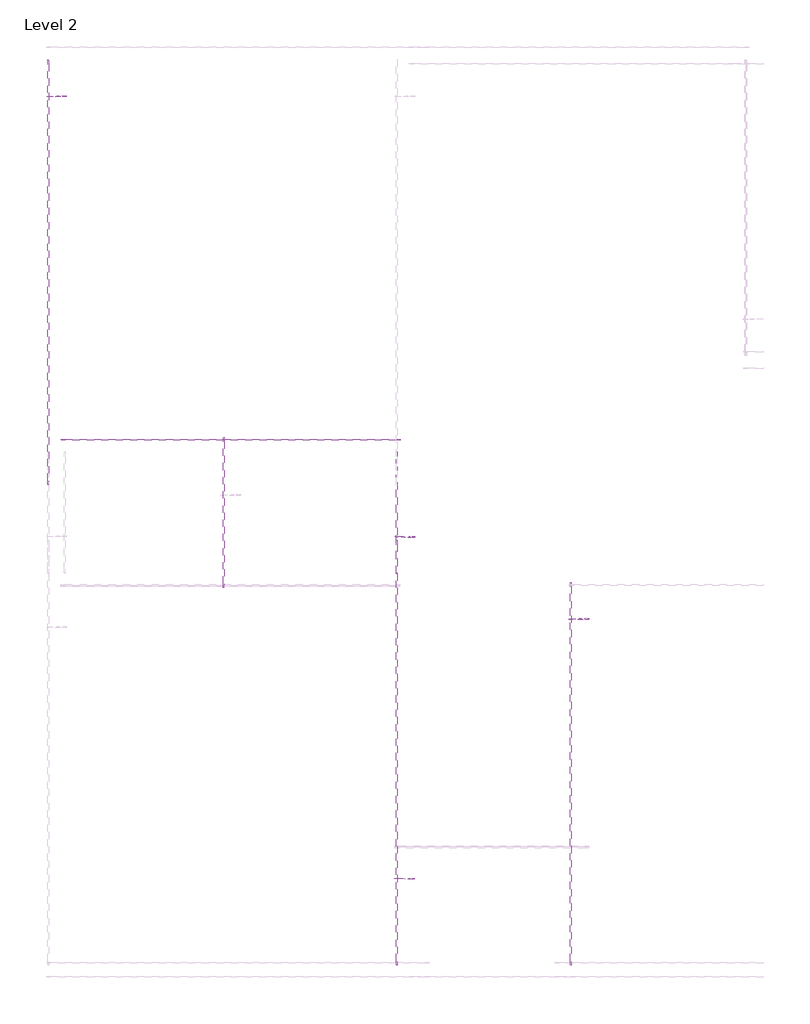
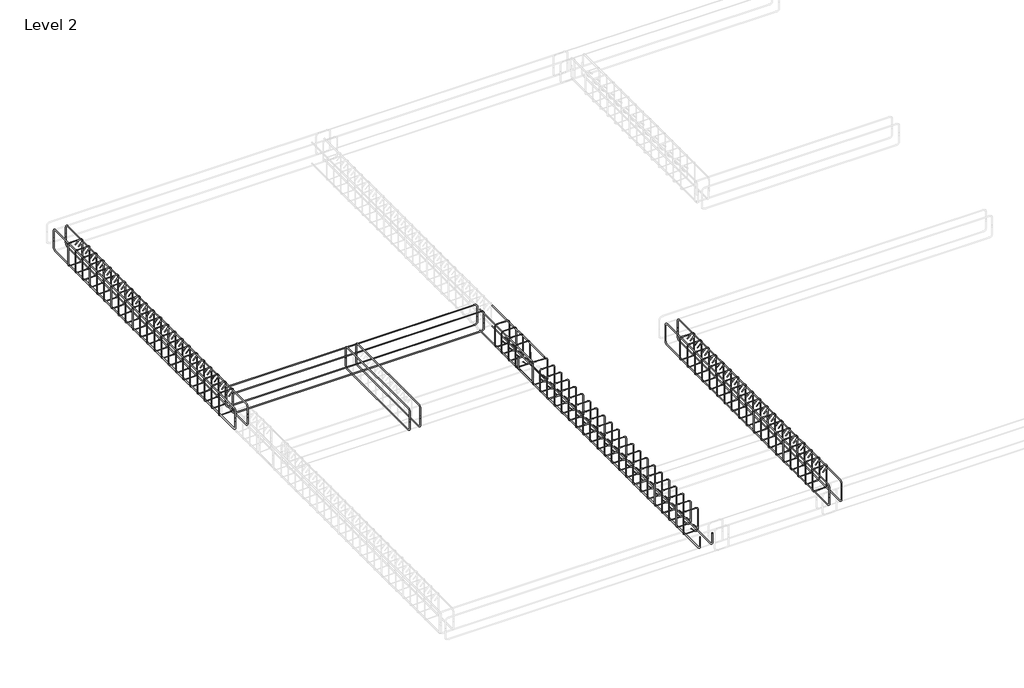
# One storey, part 3 of 5: 15 reinforcing bars.
"""IFC4 building model written with IfcOpenShell, lengths in millimetres."""

from ifc_helpers import new_model, si_unit, point, frame, origin, place, context, project, spatial, polyline, circle_curve, trimmed, segment, composite_curve, source, transform, mapped, element, save
from ifc_brep_helpers import swept_disk

model = new_model("IFC4")

# Units and contexts
model_context = context("Model", 3, world=origin())
ifc_project = project(units=[si_unit("LENGTHUNIT", "METRE", prefix="MILLI")], contexts=[model_context])

# Site, building, storey
site = spatial("IfcSite", under=ifc_project)
building = spatial("IfcBuilding", under=site)
storey = spatial("IfcBuildingStorey", under=building, Name="Level 2", Elevation=3048.0)

# Reinforcing bars
placement = place(None, origin())
reinforcing_bar_shape = source(origin(), model_context, "Body", "SolidModel", [
    swept_disk(composite_curve([segment(polyline([(-15212.455746, 8321.0577522, 5841.8967919), (-15212.455746, 8321.0577522, 5994.2967919)]), True, "CONTINUOUS"), segment(trimmed(circle_curve(frame((-15212.455746, 8276.9887522, 5994.2967919), z_axis=(1.0, 0.0, 0.0), x_axis=(0.0, 44.068999999999505, 0.0)), 44.069), [point((-15212.455746, 8321.0577522, 5994.2967919))], [point((-15212.455746, 8276.9887522, 6038.3657919))], True, "CARTESIAN"), True, "CONTINUOUS"), segment(polyline([(-15212.455746, 8276.9887522, 6038.3657919), (-15212.455746, 3496.0647522, 6038.3657919)]), True, "CONTINUOUS"), segment(trimmed(circle_curve(frame((-15212.455746, 3496.0647522, 5994.2967919), z_axis=(1.0, 0.0, 0.0), x_axis=(0.0, 0.0, 44.068999999999505)), 44.069), [point((-15212.455746, 3496.0647522, 6038.3657919))], [point((-15212.455746, 3451.9957522, 5994.2967919))], True, "CARTESIAN"), True, "CONTINUOUS"), segment(polyline([(-15212.455746, 3451.9957522, 5994.2967919), (-15212.455746, 3451.9957522, 5841.8967919)]), True, "CONTINUOUS")], self_intersect=False), 5.969),
])
element("IfcReinforcingBar", 1, at=placement, inside=storey, context=model_context, shape_type="MappedRepresentation", body=[
    mapped(reinforcing_bar_shape, transform((0.0, 0.0, 0.0), x_axis=(1.0, 0.0, 0.0), y_axis=(0.0, 1.0, 0.0), z_axis=(0.0, 0.0, 1.0))),
    mapped(reinforcing_bar_shape, transform((-189.5315837, 0.0, 0.0), x_axis=(1.0, 0.0, 0.0), y_axis=(0.0, 1.0, 0.0), z_axis=(0.0, 0.0, 1.0))),
])
reinforcing_bar_2_shape = source(origin(), model_context, "Body", "SolidModel", [
    swept_disk(composite_curve([segment(polyline([(-15212.455746, 3451.9957522, 5892.9032081), (-15212.455746, 3451.9957522, 5740.5032081)]), True, "CONTINUOUS"), segment(trimmed(circle_curve(frame((-15212.455746, 3496.0647522, 5740.5032081), z_axis=(1.0, 0.0, 0.0), x_axis=(0.0, -44.06899999999996, 0.0)), 44.069), [point((-15212.455746, 3451.9957522, 5740.5032081))], [point((-15212.455746, 3496.0647522, 5696.4342081))], True, "CARTESIAN"), True, "CONTINUOUS"), segment(polyline([(-15212.455746, 3496.0647522, 5696.4342081), (-15212.455746, 8276.9887522, 5696.4342081)]), True, "CONTINUOUS"), segment(trimmed(circle_curve(frame((-15212.455746, 8276.9887522, 5740.5032081), z_axis=(1.0, 0.0, 0.0), x_axis=(0.0, 0.0, -44.068999999999505)), 44.069), [point((-15212.455746, 8276.9887522, 5696.4342081))], [point((-15212.455746, 8321.0577522, 5740.5032081))], True, "CARTESIAN"), True, "CONTINUOUS"), segment(polyline([(-15212.455746, 8321.0577522, 5740.5032081), (-15212.455746, 8321.0577522, 5892.9032081)]), True, "CONTINUOUS")], self_intersect=False), 5.969),
])
element("IfcReinforcingBar", 2, at=placement, inside=storey, context=model_context, shape_type="MappedRepresentation", body=[
    mapped(reinforcing_bar_2_shape, transform((0.0, 0.0, 0.0), x_axis=(1.0, 0.0, 0.0), y_axis=(0.0, 1.0, 0.0), z_axis=(0.0, 0.0, 1.0))),
    mapped(reinforcing_bar_2_shape, transform((-189.5315837, 0.0, 0.0), x_axis=(1.0, 0.0, 0.0), y_axis=(0.0, 1.0, 0.0), z_axis=(0.0, 0.0, 1.0))),
])
reinforcing_bar_3_shape = source(origin(), model_context, "Body", "SolidModel", [
    swept_disk(composite_curve([segment(polyline([(-15260.3161447, 7903.9897522, 5949.0166099), (-15205.4511463, 7903.9897522, 6003.8816084)]), True, "CONTINUOUS"), segment(trimmed(circle_curve(frame((-15226.1955379, 7903.9897522, 6024.626), z_axis=(0.0, -1.0, 0.0), x_axis=(20.74439159999929, 0.0, -20.7443916000002)), 29.337), [point((-15205.4511463, 7903.9897522, 6003.8816084))], [point((-15226.1955379, 7903.9897522, 6053.963))], True, "CARTESIAN"), True, "CONTINUOUS"), segment(polyline([(-15226.1955379, 7903.9897522, 6053.963), (-15388.2475379, 7903.9897522, 6053.963)]), True, "CONTINUOUS"), segment(trimmed(circle_curve(frame((-15388.2475379, 7903.9897522, 6024.626), z_axis=(0.0, -1.0, 0.0), x_axis=(0.0, 0.0, 29.336999999999534)), 29.337), [point((-15388.2475379, 7903.9897522, 6053.963))], [point((-15417.5845379, 7903.9897522, 6024.626))], True, "CARTESIAN"), True, "CONTINUOUS"), segment(polyline([(-15417.5845379, 7903.9897522, 6024.626), (-15417.5845379, 7903.9897522, 5710.174)]), True, "CONTINUOUS"), segment(trimmed(circle_curve(frame((-15388.2661869, 7905.0356312, 5710.174), z_axis=(0.03565051078635043, -0.9993643184948482, 0.0), x_axis=(-29.318350999999893, -1.045879000000241, 0.0)), 29.337), [point((-15417.5845379, 7903.9897522, 5710.174))], [point((-15388.2661869, 7905.0356312, 5680.837))], True, "CARTESIAN"), True, "CONTINUOUS"), segment(polyline([(-15388.2661869, 7905.0356312, 5680.837), (-15226.1768889, 7910.8178731, 5680.837)]), True, "CONTINUOUS"), segment(trimmed(circle_curve(frame((-15226.1768889, 7910.8178731, 5710.174), z_axis=(0.03565051078635043, -0.9993643184948482, 0.0), x_axis=(0.0, 0.0, -29.336999999999534)), 29.337), [point((-15226.1768889, 7910.8178731, 5680.837))], [point((-15196.8585379, 7911.8637522, 5710.174))], True, "CARTESIAN"), True, "CONTINUOUS"), segment(polyline([(-15196.8585379, 7911.8637522, 5710.174), (-15196.8585379, 7911.8637522, 6024.626)]), True, "CONTINUOUS"), segment(trimmed(circle_curve(frame((-15226.1955379, 7911.8637522, 6024.626), z_axis=(0.0, -1.0, 0.0), x_axis=(29.336999999999534, 0.0, 0.0)), 29.337), [point((-15196.8585379, 7911.8637522, 6024.626))], [point((-15246.9399295, 7911.8637522, 6045.3703916))], True, "CARTESIAN"), True, "CONTINUOUS"), segment(polyline([(-15246.9399295, 7911.8637522, 6045.3703916), (-15301.804928, 7911.8637522, 5990.5053932)]), True, "CONTINUOUS")], self_intersect=False), 3.937),
])
element("IfcReinforcingBar", 3, at=placement, inside=storey, context=model_context, shape_type="MappedRepresentation", body=[
    mapped(reinforcing_bar_3_shape, transform((0.0, 0.0, 0.0), x_axis=(1.0, 0.0, 0.0), y_axis=(0.0, 1.0, 0.0), z_axis=(0.0, 0.0, 1.0))),
    mapped(reinforcing_bar_3_shape, transform((0.0, -192.1393333, 0.0), x_axis=(1.0, 0.0, 0.0), y_axis=(0.0, 1.0, 0.0), z_axis=(0.0, 0.0, 1.0))),
    mapped(reinforcing_bar_3_shape, transform((0.0, -384.2786667, 0.0), x_axis=(1.0, 0.0, 0.0), y_axis=(0.0, 1.0, 0.0), z_axis=(0.0, 0.0, 1.0))),
    mapped(reinforcing_bar_3_shape, transform((0.0, -576.418, 0.0), x_axis=(1.0, 0.0, 0.0), y_axis=(0.0, 1.0, 0.0), z_axis=(0.0, 0.0, 1.0))),
    mapped(reinforcing_bar_3_shape, transform((0.0, -768.5573333, 0.0), x_axis=(1.0, 0.0, 0.0), y_axis=(0.0, 1.0, 0.0), z_axis=(0.0, 0.0, 1.0))),
    mapped(reinforcing_bar_3_shape, transform((0.0, -960.6966667, 0.0), x_axis=(1.0, 0.0, 0.0), y_axis=(0.0, 1.0, 0.0), z_axis=(0.0, 0.0, 1.0))),
    mapped(reinforcing_bar_3_shape, transform((0.0, -1152.836, 0.0), x_axis=(1.0, 0.0, 0.0), y_axis=(0.0, 1.0, 0.0), z_axis=(0.0, 0.0, 1.0))),
    mapped(reinforcing_bar_3_shape, transform((0.0, -1344.9753333, 0.0), x_axis=(1.0, 0.0, 0.0), y_axis=(0.0, 1.0, 0.0), z_axis=(0.0, 0.0, 1.0))),
    mapped(reinforcing_bar_3_shape, transform((0.0, -1537.1146667, 0.0), x_axis=(1.0, 0.0, 0.0), y_axis=(0.0, 1.0, 0.0), z_axis=(0.0, 0.0, 1.0))),
    mapped(reinforcing_bar_3_shape, transform((0.0, -1729.254, 0.0), x_axis=(1.0, 0.0, 0.0), y_axis=(0.0, 1.0, 0.0), z_axis=(0.0, 0.0, 1.0))),
    mapped(reinforcing_bar_3_shape, transform((0.0, -1921.3933333, 0.0), x_axis=(1.0, 0.0, 0.0), y_axis=(0.0, 1.0, 0.0), z_axis=(0.0, 0.0, 1.0))),
    mapped(reinforcing_bar_3_shape, transform((0.0, -2113.5326667, 0.0), x_axis=(1.0, 0.0, 0.0), y_axis=(0.0, 1.0, 0.0), z_axis=(0.0, 0.0, 1.0))),
    mapped(reinforcing_bar_3_shape, transform((0.0, -2305.672, 0.0), x_axis=(1.0, 0.0, 0.0), y_axis=(0.0, 1.0, 0.0), z_axis=(0.0, 0.0, 1.0))),
    mapped(reinforcing_bar_3_shape, transform((0.0, -2497.8113333, 0.0), x_axis=(1.0, 0.0, 0.0), y_axis=(0.0, 1.0, 0.0), z_axis=(0.0, 0.0, 1.0))),
    mapped(reinforcing_bar_3_shape, transform((0.0, -2689.9506667, 0.0), x_axis=(1.0, 0.0, 0.0), y_axis=(0.0, 1.0, 0.0), z_axis=(0.0, 0.0, 1.0))),
    mapped(reinforcing_bar_3_shape, transform((0.0, -2882.09, 0.0), x_axis=(1.0, 0.0, 0.0), y_axis=(0.0, 1.0, 0.0), z_axis=(0.0, 0.0, 1.0))),
    mapped(reinforcing_bar_3_shape, transform((0.0, -3074.2293333, 0.0), x_axis=(1.0, 0.0, 0.0), y_axis=(0.0, 1.0, 0.0), z_axis=(0.0, 0.0, 1.0))),
    mapped(reinforcing_bar_3_shape, transform((0.0, -3266.3686667, 0.0), x_axis=(1.0, 0.0, 0.0), y_axis=(0.0, 1.0, 0.0), z_axis=(0.0, 0.0, 1.0))),
    mapped(reinforcing_bar_3_shape, transform((0.0, -3458.508, 0.0), x_axis=(1.0, 0.0, 0.0), y_axis=(0.0, 1.0, 0.0), z_axis=(0.0, 0.0, 1.0))),
    mapped(reinforcing_bar_3_shape, transform((0.0, -3650.6473333, 0.0), x_axis=(1.0, 0.0, 0.0), y_axis=(0.0, 1.0, 0.0), z_axis=(0.0, 0.0, 1.0))),
    mapped(reinforcing_bar_3_shape, transform((0.0, -3842.7866667, 0.0), x_axis=(1.0, 0.0, 0.0), y_axis=(0.0, 1.0, 0.0), z_axis=(0.0, 0.0, 1.0))),
    mapped(reinforcing_bar_3_shape, transform((0.0, -4034.926, 0.0), x_axis=(1.0, 0.0, 0.0), y_axis=(0.0, 1.0, 0.0), z_axis=(0.0, 0.0, 1.0))),
])
reinforcing_bar_4_shape = source(origin(), model_context, "Body", "SolidModel", [
    swept_disk(composite_curve([segment(polyline([(-13226.1955379, 3986.1577522, 5847.588), (-13226.1955379, 3986.1577522, 5999.988)]), True, "CONTINUOUS"), segment(trimmed(circle_curve(frame((-13226.1955379, 3942.0887522, 5999.988), z_axis=(1.0, 0.0, 0.0), x_axis=(0.0, 44.06899999999996, 0.0)), 44.069), [point((-13226.1955379, 3986.1577522, 5999.988))], [point((-13226.1955379, 3942.0887522, 6044.057))], True, "CARTESIAN"), True, "CONTINUOUS"), segment(polyline([(-13226.1955379, 3942.0887522, 6044.057), (-13226.1955379, 2313.5647522, 6044.057)]), True, "CONTINUOUS"), segment(trimmed(circle_curve(frame((-13226.1955379, 2313.5647522, 5999.988), z_axis=(1.0, 0.0, 0.0), x_axis=(0.0, 0.0, 44.068999999999505)), 44.069), [point((-13226.1955379, 2313.5647522, 6044.057))], [point((-13226.1955379, 2269.4957522, 5999.988))], True, "CARTESIAN"), True, "CONTINUOUS"), segment(polyline([(-13226.1955379, 2269.4957522, 5999.988), (-13226.1955379, 2269.4957522, 5847.588)]), True, "CONTINUOUS")], self_intersect=False), 5.969),
])
element("IfcReinforcingBar", 4, at=placement, inside=storey, context=model_context, shape_type="MappedRepresentation", body=[
    mapped(reinforcing_bar_4_shape, transform((0.0, 0.0, 0.0), x_axis=(1.0, 0.0, 0.0), y_axis=(0.0, 1.0, 0.0), z_axis=(0.0, 0.0, 1.0))),
    mapped(reinforcing_bar_4_shape, transform((-162.052, 0.0, 0.0), x_axis=(1.0, 0.0, 0.0), y_axis=(0.0, 1.0, 0.0), z_axis=(0.0, 0.0, 1.0))),
])
reinforcing_bar_5_shape = source(origin(), model_context, "Body", "SolidModel", [
    swept_disk(composite_curve([segment(polyline([(-13388.2475379, 2269.4957522, 5887.212), (-13388.2475379, 2269.4957522, 5734.812)]), True, "CONTINUOUS"), segment(trimmed(circle_curve(frame((-13388.2475379, 2313.5647522, 5734.812), z_axis=(1.0, 0.0, 0.0), x_axis=(0.0, -44.06899999999996, 0.0)), 44.069), [point((-13388.2475379, 2269.4957522, 5734.812))], [point((-13388.2475379, 2313.5647522, 5690.743))], True, "CARTESIAN"), True, "CONTINUOUS"), segment(polyline([(-13388.2475379, 2313.5647522, 5690.743), (-13388.2475379, 3942.0887522, 5690.743)]), True, "CONTINUOUS"), segment(trimmed(circle_curve(frame((-13388.2475379, 3942.0887522, 5734.812), z_axis=(1.0, 0.0, 0.0), x_axis=(0.0, 0.0, -44.068999999999505)), 44.069), [point((-13388.2475379, 3942.0887522, 5690.743))], [point((-13388.2475379, 3986.1577522, 5734.812))], True, "CARTESIAN"), True, "CONTINUOUS"), segment(polyline([(-13388.2475379, 3986.1577522, 5734.812), (-13388.2475379, 3986.1577522, 5887.212)]), True, "CONTINUOUS")], self_intersect=False), 5.969),
])
element("IfcReinforcingBar", 5, at=placement, inside=storey, context=model_context, shape_type="MappedRepresentation", body=[
    mapped(reinforcing_bar_5_shape, transform((0.0, 0.0, 0.0), x_axis=(1.0, 0.0, 0.0), y_axis=(0.0, 1.0, 0.0), z_axis=(0.0, 0.0, 1.0))),
    mapped(reinforcing_bar_5_shape, transform((162.052, 0.0, 0.0), x_axis=(1.0, 0.0, 0.0), y_axis=(0.0, 1.0, 0.0), z_axis=(0.0, 0.0, 1.0))),
])
reinforcing_bar_6_shape = source(origin(), model_context, "Body", "SolidModel", [
    swept_disk(composite_curve([segment(polyline([(-15250.4525379, 3964.464544, 5833.7687919), (-15250.4525379, 3964.464544, 5986.1687919)]), True, "CONTINUOUS"), segment(trimmed(circle_curve(frame((-15206.3835379, 3964.464544, 5986.1687919), z_axis=(0.0, 1.0, 0.0), x_axis=(-44.069000000001324, 0.0, 0.0)), 44.069), [point((-15250.4525379, 3964.464544, 5986.1687919))], [point((-15206.3835379, 3964.464544, 6030.2377919))], True, "CARTESIAN"), True, "CONTINUOUS"), segment(polyline([(-15206.3835379, 3964.464544, 6030.2377919), (-11408.0595379, 3964.464544, 6030.2377919)]), True, "CONTINUOUS"), segment(trimmed(circle_curve(frame((-11408.0595379, 3964.464544, 5986.1687919), z_axis=(0.0, 1.0, 0.0), x_axis=(0.0, 0.0, 44.069000000000415)), 44.069), [point((-11408.0595379, 3964.464544, 6030.2377919))], [point((-11363.9905379, 3964.464544, 5986.1687919))], True, "CARTESIAN"), True, "CONTINUOUS"), segment(polyline([(-11363.9905379, 3964.464544, 5986.1687919), (-11363.9905379, 3964.464544, 5833.7687919)]), True, "CONTINUOUS")], self_intersect=False), 5.969),
])
element("IfcReinforcingBar", 6, at=placement, inside=storey, context=model_context, shape_type="MappedRepresentation", body=[
    mapped(reinforcing_bar_6_shape, transform((0.0, 0.0, 0.0), x_axis=(1.0, 0.0, 0.0), y_axis=(0.0, 1.0, 0.0), z_axis=(0.0, 0.0, 1.0))),
    mapped(reinforcing_bar_6_shape, transform((0.0, -173.2755837, 0.0), x_axis=(1.0, 0.0, 0.0), y_axis=(0.0, 1.0, 0.0), z_axis=(0.0, 0.0, 1.0))),
])
reinforcing_bar_7_shape = source(origin(), model_context, "Body", "SolidModel", [
    swept_disk(composite_curve([segment(polyline([(-11363.9905379, 3964.464544, 5901.0312081), (-11363.9905379, 3964.464544, 5748.6312081)]), True, "CONTINUOUS"), segment(trimmed(circle_curve(frame((-11408.0595379, 3964.464544, 5748.6312081), z_axis=(0.0, 1.0, 0.0), x_axis=(44.069000000001324, 0.0, 0.0)), 44.069), [point((-11363.9905379, 3964.464544, 5748.6312081))], [point((-11408.0595379, 3964.464544, 5704.5622081))], True, "CARTESIAN"), True, "CONTINUOUS"), segment(polyline([(-11408.0595379, 3964.464544, 5704.5622081), (-15206.3835379, 3964.464544, 5704.5622081)]), True, "CONTINUOUS"), segment(trimmed(circle_curve(frame((-15206.3835379, 3964.464544, 5748.6312081), z_axis=(0.0, 1.0, 0.0), x_axis=(0.0, 0.0, -44.068999999999505)), 44.069), [point((-15206.3835379, 3964.464544, 5704.5622081))], [point((-15250.4525379, 3964.464544, 5748.6312081))], True, "CARTESIAN"), True, "CONTINUOUS"), segment(polyline([(-15250.4525379, 3964.464544, 5748.6312081), (-15250.4525379, 3964.464544, 5901.0312081)]), True, "CONTINUOUS")], self_intersect=False), 5.969),
])
element("IfcReinforcingBar", 7, at=placement, inside=storey, context=model_context, shape_type="MappedRepresentation", body=[
    mapped(reinforcing_bar_7_shape, transform((0.0, 0.0, 0.0), x_axis=(1.0, 0.0, 0.0), y_axis=(0.0, 1.0, 0.0), z_axis=(0.0, 0.0, 1.0))),
    mapped(reinforcing_bar_7_shape, transform((0.0, -173.2755837, 0.0), x_axis=(1.0, 0.0, 0.0), y_axis=(0.0, 1.0, 0.0), z_axis=(0.0, 0.0, 1.0))),
])
reinforcing_bar_8_shape = source(origin(), model_context, "Body", "SolidModel", [
    swept_disk(composite_curve([segment(polyline([(-11212.455746, 3827.0267522, 6038.3657919), (-11212.455746, 2428.6267522, 6038.3657919)]), True, "CONTINUOUS")], self_intersect=False), 5.969),
])
element("IfcReinforcingBar", 8, at=placement, inside=storey, context=model_context, shape_type="MappedRepresentation", body=[
    mapped(reinforcing_bar_8_shape, transform((0.0, 0.0, 0.0), x_axis=(1.0, 0.0, 0.0), y_axis=(0.0, 1.0, 0.0), z_axis=(0.0, 0.0, 1.0))),
    mapped(reinforcing_bar_8_shape, transform((-189.5315837, 0.0, 0.0), x_axis=(1.0, 0.0, 0.0), y_axis=(0.0, 1.0, 0.0), z_axis=(0.0, 0.0, 1.0))),
])
reinforcing_bar_9_shape = source(origin(), model_context, "Body", "SolidModel", [
    swept_disk(composite_curve([segment(polyline([(-11212.455746, 2428.6267522, 5696.4342081), (-11212.455746, 3827.0267522, 5696.4342081)]), True, "CONTINUOUS")], self_intersect=False), 5.969),
])
element("IfcReinforcingBar", 9, at=placement, inside=storey, context=model_context, shape_type="MappedRepresentation", body=[
    mapped(reinforcing_bar_9_shape, transform((0.0, 0.0, 0.0), x_axis=(1.0, 0.0, 0.0), y_axis=(0.0, 1.0, 0.0), z_axis=(0.0, 0.0, 1.0))),
    mapped(reinforcing_bar_9_shape, transform((-189.5315837, 0.0, 0.0), x_axis=(1.0, 0.0, 0.0), y_axis=(0.0, 1.0, 0.0), z_axis=(0.0, 0.0, 1.0))),
])
reinforcing_bar_10_shape = source(origin(), model_context, "Body", "SolidModel", [
    swept_disk(composite_curve([segment(polyline([(-11212.455746, -2065.4042478, 5892.9032081), (-11212.455746, -2065.4042478, 5740.5032081)]), True, "CONTINUOUS"), segment(trimmed(circle_curve(frame((-11212.455746, -2021.3352478, 5740.5032081), z_axis=(1.0, 0.0, 0.0), x_axis=(0.0, -44.06900000000019, 0.0)), 44.069), [point((-11212.455746, -2065.4042478, 5740.5032081))], [point((-11212.455746, -2021.3352478, 5696.4342081))], True, "CARTESIAN"), True, "CONTINUOUS"), segment(polyline([(-11212.455746, -2021.3352478, 5696.4342081), (-11212.455746, 2759.5887522, 5696.4342081)]), True, "CONTINUOUS"), segment(trimmed(circle_curve(frame((-11212.455746, 2759.5887522, 5740.5032081), z_axis=(1.0, 0.0, 0.0), x_axis=(0.0, 0.0, -44.068999999999505)), 44.069), [point((-11212.455746, 2759.5887522, 5696.4342081))], [point((-11212.455746, 2803.6577522, 5740.5032081))], True, "CARTESIAN"), True, "CONTINUOUS"), segment(polyline([(-11212.455746, 2803.6577522, 5740.5032081), (-11212.455746, 2803.6577522, 5892.9032081)]), True, "CONTINUOUS")], self_intersect=False), 5.969),
])
element("IfcReinforcingBar", 10, at=placement, inside=storey, context=model_context, shape_type="MappedRepresentation", body=[
    mapped(reinforcing_bar_10_shape, transform((0.0, 0.0, 0.0), x_axis=(1.0, 0.0, 0.0), y_axis=(0.0, 1.0, 0.0), z_axis=(0.0, 0.0, 1.0))),
    mapped(reinforcing_bar_10_shape, transform((-189.5315837, 0.0, 0.0), x_axis=(1.0, 0.0, 0.0), y_axis=(0.0, 1.0, 0.0), z_axis=(0.0, 0.0, 1.0))),
])
reinforcing_bar_11_shape = source(origin(), model_context, "Body", "SolidModel", [
    swept_disk(composite_curve([segment(polyline([(-11260.3161447, -1648.3362478, 5785.7833901), (-11205.4511463, -1648.3362478, 5730.9183916)]), True, "CONTINUOUS"), segment(trimmed(circle_curve(frame((-11226.1955379, -1648.3362478, 5710.174), z_axis=(0.0, 1.0, 0.0), x_axis=(20.74439159999929, 0.0, 20.7443916000002)), 29.337), [point((-11205.4511463, -1648.3362478, 5730.9183916))], [point((-11226.1955379, -1648.3362478, 5680.837))], True, "CARTESIAN"), True, "CONTINUOUS"), segment(polyline([(-11226.1955379, -1648.3362478, 5680.837), (-11388.2475379, -1648.3362478, 5680.837)]), True, "CONTINUOUS"), segment(trimmed(circle_curve(frame((-11388.2475379, -1648.3362478, 5710.174), z_axis=(0.0, 1.0, 0.0), x_axis=(0.0, 0.0, -29.336999999999534)), 29.337), [point((-11388.2475379, -1648.3362478, 5680.837))], [point((-11417.5845379, -1648.3362478, 5710.174))], True, "CARTESIAN"), True, "CONTINUOUS"), segment(polyline([(-11417.5845379, -1648.3362478, 5710.174), (-11417.5845379, -1648.3362478, 6024.626)]), True, "CONTINUOUS"), segment(trimmed(circle_curve(frame((-11388.2661869, -1649.3821269, 6024.626), z_axis=(0.03565051078635425, 0.9993643184948481, 0.0), x_axis=(-29.318350999999893, 1.0458791000000929, 0.0)), 29.337), [point((-11417.5845379, -1648.3362478, 6024.626))], [point((-11388.2661869, -1649.3821269, 6053.963))], True, "CARTESIAN"), True, "CONTINUOUS"), segment(polyline([(-11388.2661869, -1649.3821269, 6053.963), (-11226.1768889, -1655.1643688, 6053.963)]), True, "CONTINUOUS"), segment(trimmed(circle_curve(frame((-11226.1768889, -1655.1643688, 6024.626), z_axis=(0.03565051078635425, 0.9993643184948481, 0.0), x_axis=(0.0, 0.0, 29.336999999999534)), 29.337), [point((-11226.1768889, -1655.1643688, 6053.963))], [point((-11196.8585379, -1656.2102478, 6024.626))], True, "CARTESIAN"), True, "CONTINUOUS"), segment(polyline([(-11196.8585379, -1656.2102478, 6024.626), (-11196.8585379, -1656.2102478, 5710.174)]), True, "CONTINUOUS"), segment(trimmed(circle_curve(frame((-11226.1955379, -1656.2102478, 5710.174), z_axis=(0.0, 1.0, 0.0), x_axis=(29.336999999999534, 0.0, 0.0)), 29.337), [point((-11196.8585379, -1656.2102478, 5710.174))], [point((-11246.9399295, -1656.2102478, 5689.4296084))], True, "CARTESIAN"), True, "CONTINUOUS"), segment(polyline([(-11246.9399295, -1656.2102478, 5689.4296084), (-11301.804928, -1656.2102478, 5744.2946068)]), True, "CONTINUOUS")], self_intersect=False), 3.937),
])
element("IfcReinforcingBar", 11, at=placement, inside=storey, context=model_context, shape_type="MappedRepresentation", body=[
    mapped(reinforcing_bar_11_shape, transform((0.0, 0.0, 0.0), x_axis=(1.0, 0.0, 0.0), y_axis=(0.0, 1.0, 0.0), z_axis=(0.0, 0.0, 1.0))),
    mapped(reinforcing_bar_11_shape, transform((0.0, 192.1393333, 0.0), x_axis=(1.0, 0.0, 0.0), y_axis=(0.0, 1.0, 0.0), z_axis=(0.0, 0.0, 1.0))),
    mapped(reinforcing_bar_11_shape, transform((0.0, 384.2786667, 0.0), x_axis=(1.0, 0.0, 0.0), y_axis=(0.0, 1.0, 0.0), z_axis=(0.0, 0.0, 1.0))),
    mapped(reinforcing_bar_11_shape, transform((0.0, 576.418, 0.0), x_axis=(1.0, 0.0, 0.0), y_axis=(0.0, 1.0, 0.0), z_axis=(0.0, 0.0, 1.0))),
    mapped(reinforcing_bar_11_shape, transform((0.0, 768.5573333, 0.0), x_axis=(1.0, 0.0, 0.0), y_axis=(0.0, 1.0, 0.0), z_axis=(0.0, 0.0, 1.0))),
    mapped(reinforcing_bar_11_shape, transform((0.0, 960.6966667, 0.0), x_axis=(1.0, 0.0, 0.0), y_axis=(0.0, 1.0, 0.0), z_axis=(0.0, 0.0, 1.0))),
    mapped(reinforcing_bar_11_shape, transform((0.0, 1152.836, 0.0), x_axis=(1.0, 0.0, 0.0), y_axis=(0.0, 1.0, 0.0), z_axis=(0.0, 0.0, 1.0))),
    mapped(reinforcing_bar_11_shape, transform((0.0, 1344.9753333, 0.0), x_axis=(1.0, 0.0, 0.0), y_axis=(0.0, 1.0, 0.0), z_axis=(0.0, 0.0, 1.0))),
    mapped(reinforcing_bar_11_shape, transform((0.0, 1537.1146667, 0.0), x_axis=(1.0, 0.0, 0.0), y_axis=(0.0, 1.0, 0.0), z_axis=(0.0, 0.0, 1.0))),
    mapped(reinforcing_bar_11_shape, transform((0.0, 1729.254, 0.0), x_axis=(1.0, 0.0, 0.0), y_axis=(0.0, 1.0, 0.0), z_axis=(0.0, 0.0, 1.0))),
    mapped(reinforcing_bar_11_shape, transform((0.0, 1921.3933333, 0.0), x_axis=(1.0, 0.0, 0.0), y_axis=(0.0, 1.0, 0.0), z_axis=(0.0, 0.0, 1.0))),
    mapped(reinforcing_bar_11_shape, transform((0.0, 2113.5326667, 0.0), x_axis=(1.0, 0.0, 0.0), y_axis=(0.0, 1.0, 0.0), z_axis=(0.0, 0.0, 1.0))),
    mapped(reinforcing_bar_11_shape, transform((0.0, 2305.672, 0.0), x_axis=(1.0, 0.0, 0.0), y_axis=(0.0, 1.0, 0.0), z_axis=(0.0, 0.0, 1.0))),
    mapped(reinforcing_bar_11_shape, transform((0.0, 2497.8113333, 0.0), x_axis=(1.0, 0.0, 0.0), y_axis=(0.0, 1.0, 0.0), z_axis=(0.0, 0.0, 1.0))),
    mapped(reinforcing_bar_11_shape, transform((0.0, 2689.9506667, 0.0), x_axis=(1.0, 0.0, 0.0), y_axis=(0.0, 1.0, 0.0), z_axis=(0.0, 0.0, 1.0))),
    mapped(reinforcing_bar_11_shape, transform((0.0, 2882.09, 0.0), x_axis=(1.0, 0.0, 0.0), y_axis=(0.0, 1.0, 0.0), z_axis=(0.0, 0.0, 1.0))),
    mapped(reinforcing_bar_11_shape, transform((0.0, 3074.2293333, 0.0), x_axis=(1.0, 0.0, 0.0), y_axis=(0.0, 1.0, 0.0), z_axis=(0.0, 0.0, 1.0))),
    mapped(reinforcing_bar_11_shape, transform((0.0, 3266.3686667, 0.0), x_axis=(1.0, 0.0, 0.0), y_axis=(0.0, 1.0, 0.0), z_axis=(0.0, 0.0, 1.0))),
    mapped(reinforcing_bar_11_shape, transform((0.0, 3458.508, 0.0), x_axis=(1.0, 0.0, 0.0), y_axis=(0.0, 1.0, 0.0), z_axis=(0.0, 0.0, 1.0))),
    mapped(reinforcing_bar_11_shape, transform((0.0, 3650.6473333, 0.0), x_axis=(1.0, 0.0, 0.0), y_axis=(0.0, 1.0, 0.0), z_axis=(0.0, 0.0, 1.0))),
    mapped(reinforcing_bar_11_shape, transform((0.0, 3842.7866667, 0.0), x_axis=(1.0, 0.0, 0.0), y_axis=(0.0, 1.0, 0.0), z_axis=(0.0, 0.0, 1.0))),
    mapped(reinforcing_bar_11_shape, transform((0.0, 4034.926, 0.0), x_axis=(1.0, 0.0, 0.0), y_axis=(0.0, 1.0, 0.0), z_axis=(0.0, 0.0, 1.0))),
])
reinforcing_bar_12_shape = source(origin(), model_context, "Body", "SolidModel", [
    swept_disk(composite_curve([segment(polyline([(-11260.3161447, 2851.6637522, 5785.7833901), (-11205.4511463, 2851.6637522, 5730.9183916)]), True, "CONTINUOUS"), segment(trimmed(circle_curve(frame((-11226.1955379, 2851.6637522, 5710.174), z_axis=(0.0, 1.0, 0.0), x_axis=(20.74439159999929, 0.0, 20.7443916000002)), 29.337), [point((-11205.4511463, 2851.6637522, 5730.9183916))], [point((-11226.1955379, 2851.6637522, 5680.837))], True, "CARTESIAN"), True, "CONTINUOUS"), segment(polyline([(-11226.1955379, 2851.6637522, 5680.837), (-11388.2475379, 2851.6637522, 5680.837)]), True, "CONTINUOUS"), segment(trimmed(circle_curve(frame((-11388.2475379, 2851.6637522, 5710.174), z_axis=(0.0, 1.0, 0.0), x_axis=(0.0, 0.0, -29.336999999999534)), 29.337), [point((-11388.2475379, 2851.6637522, 5680.837))], [point((-11417.5845379, 2851.6637522, 5710.174))], True, "CARTESIAN"), True, "CONTINUOUS"), segment(polyline([(-11417.5845379, 2851.6637522, 5710.174), (-11417.5845379, 2851.6637522, 6024.626)]), True, "CONTINUOUS"), segment(trimmed(circle_curve(frame((-11388.2661869, 2850.6178731, 6024.626), z_axis=(0.03565051078635292, 0.9993643184948482, 0.0), x_axis=(-29.318350999999893, 1.0458791000000929, 0.0)), 29.337), [point((-11417.5845379, 2851.6637522, 6024.626))], [point((-11388.2661869, 2850.6178731, 6053.963))], True, "CARTESIAN"), True, "CONTINUOUS"), segment(polyline([(-11388.2661869, 2850.6178731, 6053.963), (-11226.1768889, 2844.8356312, 6053.963)]), True, "CONTINUOUS"), segment(trimmed(circle_curve(frame((-11226.1768889, 2844.8356312, 6024.626), z_axis=(0.03565051078635292, 0.9993643184948482, 0.0), x_axis=(0.0, 0.0, 29.336999999999534)), 29.337), [point((-11226.1768889, 2844.8356312, 6053.963))], [point((-11196.8585379, 2843.7897522, 6024.626))], True, "CARTESIAN"), True, "CONTINUOUS"), segment(polyline([(-11196.8585379, 2843.7897522, 6024.626), (-11196.8585379, 2843.7897522, 5710.174)]), True, "CONTINUOUS"), segment(trimmed(circle_curve(frame((-11226.1955379, 2843.7897522, 5710.174), z_axis=(0.0, 1.0, 0.0), x_axis=(29.336999999999534, 0.0, 0.0)), 29.337), [point((-11196.8585379, 2843.7897522, 5710.174))], [point((-11246.9399295, 2843.7897522, 5689.4296084))], True, "CARTESIAN"), True, "CONTINUOUS"), segment(polyline([(-11246.9399295, 2843.7897522, 5689.4296084), (-11301.804928, 2843.7897522, 5744.2946068)]), True, "CONTINUOUS")], self_intersect=False), 3.937),
])
element("IfcReinforcingBar", 12, at=placement, inside=storey, context=model_context, shape_type="MappedRepresentation", body=[
    mapped(reinforcing_bar_12_shape, transform((0.0, 0.0, 0.0), x_axis=(1.0, 0.0, 0.0), y_axis=(0.0, 1.0, 0.0), z_axis=(0.0, 0.0, 1.0))),
    mapped(reinforcing_bar_12_shape, transform((0.0, 184.1086667, 0.0), x_axis=(1.0, 0.0, 0.0), y_axis=(0.0, 1.0, 0.0), z_axis=(0.0, 0.0, 1.0))),
    mapped(reinforcing_bar_12_shape, transform((0.0, 368.2173333, 0.0), x_axis=(1.0, 0.0, 0.0), y_axis=(0.0, 1.0, 0.0), z_axis=(0.0, 0.0, 1.0))),
    mapped(reinforcing_bar_12_shape, transform((0.0, 552.326, 0.0), x_axis=(1.0, 0.0, 0.0), y_axis=(0.0, 1.0, 0.0), z_axis=(0.0, 0.0, 1.0))),
])
reinforcing_bar_13_shape = source(origin(), model_context, "Body", "SolidModel", [
    swept_disk(composite_curve([segment(polyline([(-9212.455746, 2321.0577522, 5841.8967919), (-9212.455746, 2321.0577522, 5994.2967919)]), True, "CONTINUOUS"), segment(trimmed(circle_curve(frame((-9212.455746, 2276.9887522, 5994.2967919), z_axis=(1.0, 0.0, 0.0), x_axis=(0.0, 44.06899999999996, 0.0)), 44.069), [point((-9212.455746, 2321.0577522, 5994.2967919))], [point((-9212.455746, 2276.9887522, 6038.3657919))], True, "CARTESIAN"), True, "CONTINUOUS"), segment(polyline([(-9212.455746, 2276.9887522, 6038.3657919), (-9212.455746, -2021.3352478, 6038.3657919)]), True, "CONTINUOUS"), segment(trimmed(circle_curve(frame((-9212.455746, -2021.3352478, 5994.2967919), z_axis=(1.0, 0.0, 0.0), x_axis=(0.0, 0.0, 44.068999999999505)), 44.069), [point((-9212.455746, -2021.3352478, 6038.3657919))], [point((-9212.455746, -2065.4042478, 5994.2967919))], True, "CARTESIAN"), True, "CONTINUOUS"), segment(polyline([(-9212.455746, -2065.4042478, 5994.2967919), (-9212.455746, -2065.4042478, 5841.8967919)]), True, "CONTINUOUS")], self_intersect=False), 5.969),
])
element("IfcReinforcingBar", 13, at=placement, inside=storey, context=model_context, shape_type="MappedRepresentation", body=[
    mapped(reinforcing_bar_13_shape, transform((0.0, 0.0, 0.0), x_axis=(1.0, 0.0, 0.0), y_axis=(0.0, 1.0, 0.0), z_axis=(0.0, 0.0, 1.0))),
    mapped(reinforcing_bar_13_shape, transform((-189.5315837, 0.0, 0.0), x_axis=(1.0, 0.0, 0.0), y_axis=(0.0, 1.0, 0.0), z_axis=(0.0, 0.0, 1.0))),
])
reinforcing_bar_14_shape = source(origin(), model_context, "Body", "SolidModel", [
    swept_disk(composite_curve([segment(polyline([(-9212.455746, -2065.4042478, 5892.9032081), (-9212.455746, -2065.4042478, 5740.5032081)]), True, "CONTINUOUS"), segment(trimmed(circle_curve(frame((-9212.455746, -2021.3352478, 5740.5032081), z_axis=(1.0, 0.0, 0.0), x_axis=(0.0, -44.06900000000019, 0.0)), 44.069), [point((-9212.455746, -2065.4042478, 5740.5032081))], [point((-9212.455746, -2021.3352478, 5696.4342081))], True, "CARTESIAN"), True, "CONTINUOUS"), segment(polyline([(-9212.455746, -2021.3352478, 5696.4342081), (-9212.455746, 2276.9887522, 5696.4342081)]), True, "CONTINUOUS"), segment(trimmed(circle_curve(frame((-9212.455746, 2276.9887522, 5740.5032081), z_axis=(1.0, 0.0, 0.0), x_axis=(0.0, 0.0, -44.068999999999505)), 44.069), [point((-9212.455746, 2276.9887522, 5696.4342081))], [point((-9212.455746, 2321.0577522, 5740.5032081))], True, "CARTESIAN"), True, "CONTINUOUS"), segment(polyline([(-9212.455746, 2321.0577522, 5740.5032081), (-9212.455746, 2321.0577522, 5892.9032081)]), True, "CONTINUOUS")], self_intersect=False), 5.969),
])
element("IfcReinforcingBar", 14, at=placement, inside=storey, context=model_context, shape_type="MappedRepresentation", body=[
    mapped(reinforcing_bar_14_shape, transform((0.0, 0.0, 0.0), x_axis=(1.0, 0.0, 0.0), y_axis=(0.0, 1.0, 0.0), z_axis=(0.0, 0.0, 1.0))),
    mapped(reinforcing_bar_14_shape, transform((-189.5315837, 0.0, 0.0), x_axis=(1.0, 0.0, 0.0), y_axis=(0.0, 1.0, 0.0), z_axis=(0.0, 0.0, 1.0))),
])
reinforcing_bar_15_shape = source(origin(), model_context, "Body", "SolidModel", [
    swept_disk(composite_curve([segment(polyline([(-9260.3161447, 1903.9897522, 5949.0166099), (-9205.4511463, 1903.9897522, 6003.8816084)]), True, "CONTINUOUS"), segment(trimmed(circle_curve(frame((-9226.1955379, 1903.9897522, 6024.626), z_axis=(0.0, -1.0, 0.0), x_axis=(20.74439159999929, 0.0, -20.7443916000002)), 29.337), [point((-9205.4511463, 1903.9897522, 6003.8816084))], [point((-9226.1955379, 1903.9897522, 6053.963))], True, "CARTESIAN"), True, "CONTINUOUS"), segment(polyline([(-9226.1955379, 1903.9897522, 6053.963), (-9388.2475379, 1903.9897522, 6053.963)]), True, "CONTINUOUS"), segment(trimmed(circle_curve(frame((-9388.2475379, 1903.9897522, 6024.626), z_axis=(0.0, -1.0, 0.0), x_axis=(0.0, 0.0, 29.336999999999534)), 29.337), [point((-9388.2475379, 1903.9897522, 6053.963))], [point((-9417.5845379, 1903.9897522, 6024.626))], True, "CARTESIAN"), True, "CONTINUOUS"), segment(polyline([(-9417.5845379, 1903.9897522, 6024.626), (-9417.5845379, 1903.9897522, 5710.174)]), True, "CONTINUOUS"), segment(trimmed(circle_curve(frame((-9388.2661869, 1905.0356312, 5710.174), z_axis=(0.03565051078635017, -0.9993643184948483, 0.0), x_axis=(-29.318350999999893, -1.0458789999997862, 0.0)), 29.337), [point((-9417.5845379, 1903.9897522, 5710.174))], [point((-9388.2661869, 1905.0356312, 5680.837))], True, "CARTESIAN"), True, "CONTINUOUS"), segment(polyline([(-9388.2661869, 1905.0356312, 5680.837), (-9226.1768889, 1910.8178731, 5680.837)]), True, "CONTINUOUS"), segment(trimmed(circle_curve(frame((-9226.1768889, 1910.8178731, 5710.174), z_axis=(0.03565051078635017, -0.9993643184948483, 0.0), x_axis=(0.0, 0.0, -29.336999999999534)), 29.337), [point((-9226.1768889, 1910.8178731, 5680.837))], [point((-9196.8585379, 1911.8637522, 5710.174))], True, "CARTESIAN"), True, "CONTINUOUS"), segment(polyline([(-9196.8585379, 1911.8637522, 5710.174), (-9196.8585379, 1911.8637522, 6024.626)]), True, "CONTINUOUS"), segment(trimmed(circle_curve(frame((-9226.1955379, 1911.8637522, 6024.626), z_axis=(0.0, -1.0, 0.0), x_axis=(29.336999999999534, 0.0, 0.0)), 29.337), [point((-9196.8585379, 1911.8637522, 6024.626))], [point((-9246.9399295, 1911.8637522, 6045.3703916))], True, "CARTESIAN"), True, "CONTINUOUS"), segment(polyline([(-9246.9399295, 1911.8637522, 6045.3703916), (-9301.804928, 1911.8637522, 5990.5053932)]), True, "CONTINUOUS")], self_intersect=False), 3.937),
])
element("IfcReinforcingBar", 15, at=placement, inside=storey, context=model_context, shape_type="MappedRepresentation", body=[
    mapped(reinforcing_bar_15_shape, transform((0.0, 0.0, 0.0), x_axis=(1.0, 0.0, 0.0), y_axis=(0.0, 1.0, 0.0), z_axis=(0.0, 0.0, 1.0))),
    mapped(reinforcing_bar_15_shape, transform((0.0, -197.3514444, 0.0), x_axis=(1.0, 0.0, 0.0), y_axis=(0.0, 1.0, 0.0), z_axis=(0.0, 0.0, 1.0))),
    mapped(reinforcing_bar_15_shape, transform((0.0, -394.7028889, 0.0), x_axis=(1.0, 0.0, 0.0), y_axis=(0.0, 1.0, 0.0), z_axis=(0.0, 0.0, 1.0))),
    mapped(reinforcing_bar_15_shape, transform((0.0, -592.0543333, 0.0), x_axis=(1.0, 0.0, 0.0), y_axis=(0.0, 1.0, 0.0), z_axis=(0.0, 0.0, 1.0))),
    mapped(reinforcing_bar_15_shape, transform((0.0, -789.4057778, 0.0), x_axis=(1.0, 0.0, 0.0), y_axis=(0.0, 1.0, 0.0), z_axis=(0.0, 0.0, 1.0))),
    mapped(reinforcing_bar_15_shape, transform((0.0, -986.7572222, 0.0), x_axis=(1.0, 0.0, 0.0), y_axis=(0.0, 1.0, 0.0), z_axis=(0.0, 0.0, 1.0))),
    mapped(reinforcing_bar_15_shape, transform((0.0, -1184.1086667, 0.0), x_axis=(1.0, 0.0, 0.0), y_axis=(0.0, 1.0, 0.0), z_axis=(0.0, 0.0, 1.0))),
    mapped(reinforcing_bar_15_shape, transform((0.0, -1381.4601111, 0.0), x_axis=(1.0, 0.0, 0.0), y_axis=(0.0, 1.0, 0.0), z_axis=(0.0, 0.0, 1.0))),
    mapped(reinforcing_bar_15_shape, transform((0.0, -1578.8115556, 0.0), x_axis=(1.0, 0.0, 0.0), y_axis=(0.0, 1.0, 0.0), z_axis=(0.0, 0.0, 1.0))),
    mapped(reinforcing_bar_15_shape, transform((0.0, -1776.163, 0.0), x_axis=(1.0, 0.0, 0.0), y_axis=(0.0, 1.0, 0.0), z_axis=(0.0, 0.0, 1.0))),
    mapped(reinforcing_bar_15_shape, transform((0.0, -1973.5144444, 0.0), x_axis=(1.0, 0.0, 0.0), y_axis=(0.0, 1.0, 0.0), z_axis=(0.0, 0.0, 1.0))),
    mapped(reinforcing_bar_15_shape, transform((0.0, -2170.8658889, 0.0), x_axis=(1.0, 0.0, 0.0), y_axis=(0.0, 1.0, 0.0), z_axis=(0.0, 0.0, 1.0))),
    mapped(reinforcing_bar_15_shape, transform((0.0, -2368.2173333, 0.0), x_axis=(1.0, 0.0, 0.0), y_axis=(0.0, 1.0, 0.0), z_axis=(0.0, 0.0, 1.0))),
    mapped(reinforcing_bar_15_shape, transform((0.0, -2565.5687778, 0.0), x_axis=(1.0, 0.0, 0.0), y_axis=(0.0, 1.0, 0.0), z_axis=(0.0, 0.0, 1.0))),
    mapped(reinforcing_bar_15_shape, transform((0.0, -2762.9202222, 0.0), x_axis=(1.0, 0.0, 0.0), y_axis=(0.0, 1.0, 0.0), z_axis=(0.0, 0.0, 1.0))),
    mapped(reinforcing_bar_15_shape, transform((0.0, -2960.2716667, 0.0), x_axis=(1.0, 0.0, 0.0), y_axis=(0.0, 1.0, 0.0), z_axis=(0.0, 0.0, 1.0))),
    mapped(reinforcing_bar_15_shape, transform((0.0, -3157.6231111, 0.0), x_axis=(1.0, 0.0, 0.0), y_axis=(0.0, 1.0, 0.0), z_axis=(0.0, 0.0, 1.0))),
    mapped(reinforcing_bar_15_shape, transform((0.0, -3354.9745556, 0.0), x_axis=(1.0, 0.0, 0.0), y_axis=(0.0, 1.0, 0.0), z_axis=(0.0, 0.0, 1.0))),
    mapped(reinforcing_bar_15_shape, transform((0.0, -3552.326, 0.0), x_axis=(1.0, 0.0, 0.0), y_axis=(0.0, 1.0, 0.0), z_axis=(0.0, 0.0, 1.0))),
])

save(model, "model.ifc")

# Revit data of these elements
# Elements 1, 2, 3, 4, 5, 6, 7, 8, 9, 10, 11, 12, 13, 14, 15 (IfcReinforcingBar)
#   Phase Created = New Construction
